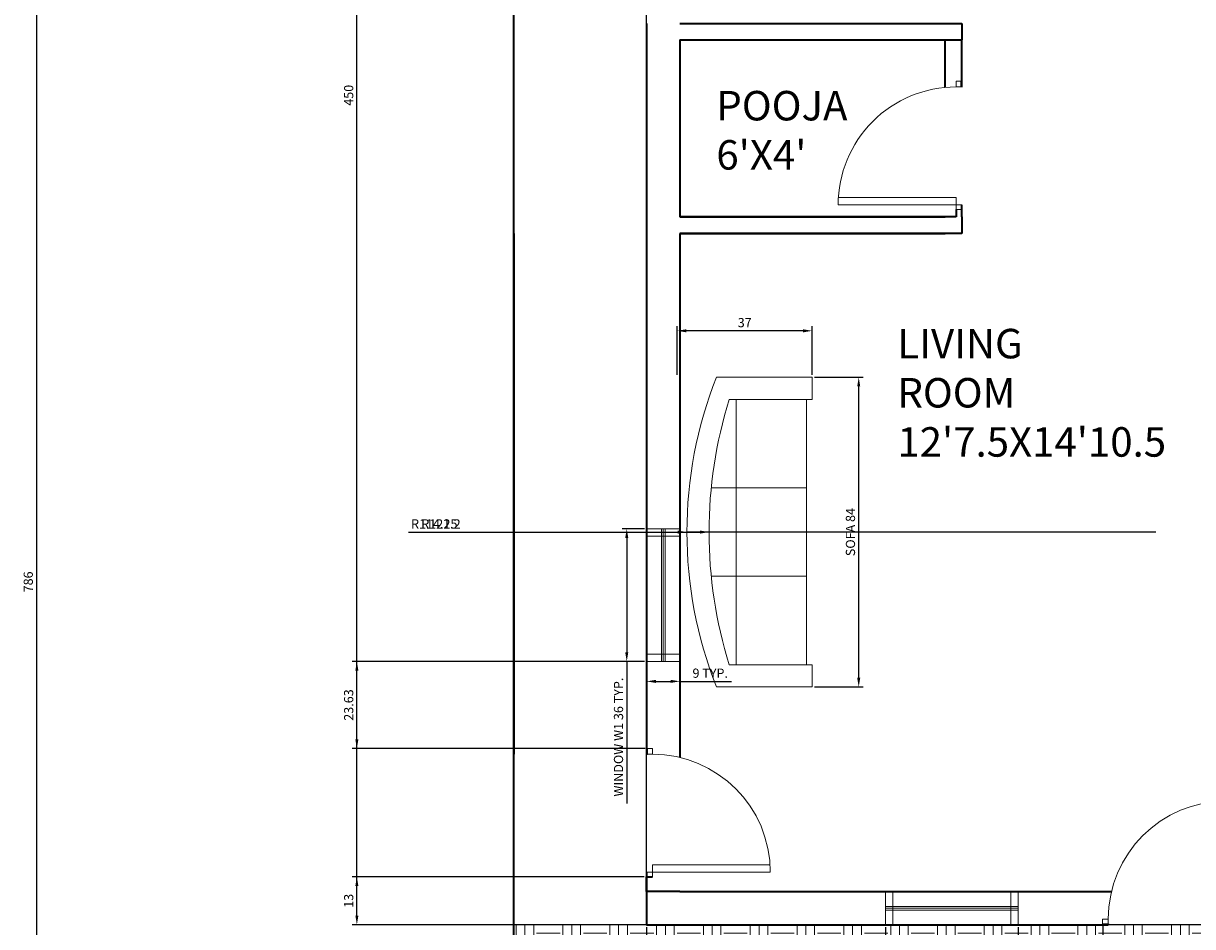
# Model space of a CAD drawing. Units: inches. Extents: x 204 to 942, y 1794 to 2670.
# Tile 3 of 6: x 204 to 521, y 2138 to 2383. Entities that reach past the tile are written whole.
import ezdxf

# ---------------------------------------------------------------- set-up
doc = ezdxf.new("R2010")
doc.units = ezdxf.units.IN
for name, color, linetype, lineweight in [('A-ANNO-DIMS', 2, 'Continuous', 18), ('A-AREA-IDEN', 7, 'Continuous', 18), ('A-DOOR', 3, 'Continuous', 18), ('A-FLOR-OTLN', 7, 'Continuous', 25), ('A-FURN', 8, 'Continuous', 18), ('A-GLAZ', 4, 'Continuous', 18), ('A-WALL', 7, 'Continuous', 35), ('C-PROP', 7, 'Continuous', 35)]:
    doc.layers.add(name, color=color, linetype=linetype, lineweight=lineweight)
doc.layers.add('A-FLOR-PATT', color=251, linetype='Continuous', lineweight=13, true_color=0x636466)
doc.styles.get("Standard").update_dxf_attribs({"font": 'arial.ttf'})
doc.dimstyles.new('ISO-25', dxfattribs={"dimtxt": 2.5, "dimasz": 2.5, "dimexe": 1.25, "dimexo": 0.625, "dimtad": 1, "dimtxsty": 'Standard', "dimcen": 2.5, "dimadec": 0, "dimazin": 0, "dimtfac": 1, "dimtmove": 0, "dimatfit": 3, "dimfxl": 1, "dimarcsym": 0})

# ---------------------------------------------------------------- blocks, each defined once
blk = doc.blocks.new('Sofa - Roundback 7 ft.')
for p, q in [((-12.00002, -32.4421), (-12.00003, -6.5971)), ((11.99997, -32.4421), (11.99998, -6.5971)), ((-36.000027, -34), (-36.000027, -11.4696)), ((35.99998, -34), (35.99998, -11.4696)), ((-35.999844, -13.3819), (35.9998, -13.3819)), ((-36.000027, -32.4421), (35.99998, -32.4421))]:
    blk.add_line(p, q)
for points in [[(-36.000027, -34), (-42.000027, -34), (-42.000027, -8)], [(41.99998, -8), (41.99998, -34), (35.99998, -34)]]:
    blk.add_lwpolyline(points)
for centre, radius, start, end in [((0, -114.25), 114.25, 68.43141, 111.5686), ((-0.00001, -127.1968), 121.1968, 72.72033, 107.2797)]:
    blk.add_arc(centre, radius, start, end)
blk = doc.blocks.new('*D11')
at = {"layer": 'A-ANNO-DIMS', "color": 0, "lineweight": -2, "transparency": 16777216}
for p, q in [((336.12, 2624.26), (205.97, 2624.26)), ((207.22, 2621.76), (207.22, 1840.76)), ((336.12, 1838.26), (205.97, 1838.26))]:
    blk.add_line(p, q, dxfattribs=at)
at = {"layer": 'A-ANNO-DIMS', "color": 0, "transparency": 16777216}
for points in [[(206.8, 2621.76), (207.63, 2621.76), (207.22, 2624.26)], [(206.8, 1840.76), (207.63, 1840.76), (207.22, 1838.26)]]:
    blk.add_solid(points, dxfattribs=at)
at = {"layer": 'Defpoints', "color": 0, "transparency": 16777216}
for p in [(336.74, 2624.26), (207.22, 1838.26), (336.74, 1838.26)]:
    blk.add_point(p, dxfattribs=at)
at = {"layer": 'A-ANNO-DIMS', "color": 0, "transparency": 16777216, "insert": (205.32, 2231.26), "char_height": 2.5, "attachment_point": 5, "rotation": 90}
blk.add_mtext('786', dxfattribs=at)
blk = doc.blocks.new('WIN-36IN')
for p, q in [((0, 9), (36, 9)), ((0, 0), (0, 9)), ((2, 0), (2, 9)), ((34, 0), (34, 9)), ((36, 9), (36, 0)), ((0, 5), (36, 5)), ((0, 4.5), (36, 4.5)), ((0, 4), (36, 4)), ((36, 0), (0, 0)), ((0, 0), (2, 0)), ((36, 0), (34, 0))]:
    blk.add_line(p, q)
blk = doc.blocks.new('DOOR-SWING-32IN')
for p, q in [((3.26, 1.55), (3.26, 33.49)), ((1.26, 1.55), (3.26, 1.55))]:
    blk.add_line(p, q)
blk.add_lwpolyline([(1.26, 33.55), (1.26, 1.55), (3.26, 1.55)])
for points in [[(1.26, 1.55), (0, 1.55), (0, 0), (1.26, 0)], [(33.26, 1.55), (34.79, 1.55), (34.79, 0.26), (33.26, 0.26)]]:
    blk.add_lwpolyline(points, close=True)
blk.add_arc((1.26, 1.55), 32, 0, 90)
blk = doc.blocks.new('*D18')
at = {"layer": 'A-ANNO-DIMS', "color": 0, "lineweight": -2, "transparency": 16777216}
for p, q in [((372.13, 2245.68), (366.1, 2245.68)), ((367.35, 2243.18), (367.35, 2212.18)), ((372.13, 2209.68), (366.1, 2209.68)), ((367.35, 2209.68), (367.35, 2171.15))]:
    blk.add_line(p, q, dxfattribs=at)
at = {"layer": 'A-ANNO-DIMS', "color": 0, "transparency": 16777216}
for points in [[(366.94, 2243.18), (367.77, 2243.18), (367.35, 2245.68)], [(366.94, 2212.18), (367.77, 2212.18), (367.35, 2209.68)]]:
    blk.add_solid(points, dxfattribs=at)
at = {"layer": 'Defpoints', "color": 0, "transparency": 16777216}
for p in [(372.75, 2245.68), (367.35, 2209.68), (372.75, 2209.68)]:
    blk.add_point(p, dxfattribs=at)
at = {"layer": 'A-ANNO-DIMS', "color": 0, "transparency": 16777216, "insert": (365.44, 2189.16), "char_height": 2.5, "attachment_point": 5, "rotation": 90}
blk.add_mtext('WINDOW W1 36 TYP.', dxfattribs=at)
blk = doc.blocks.new('*D19')
at = {"layer": 'A-ANNO-DIMS', "color": 0, "lineweight": -2, "transparency": 16777216}
for p, q in [((372.75, 2209.05), (372.75, 2203.03)), ((381.75, 2209.05), (381.75, 2203.03)), ((375.25, 2204.28), (379.25, 2204.28)), ((381.75, 2204.28), (395.73, 2204.28))]:
    blk.add_line(p, q, dxfattribs=at)
at = {"layer": 'A-ANNO-DIMS', "color": 0, "transparency": 16777216}
for points in [[(375.25, 2204.69), (375.25, 2203.86), (372.75, 2204.28)], [(379.25, 2204.69), (379.25, 2203.86), (381.75, 2204.28)]]:
    blk.add_solid(points, dxfattribs=at)
at = {"layer": 'Defpoints', "color": 0, "transparency": 16777216}
for p in [(372.75, 2209.68), (381.75, 2209.68), (381.75, 2204.28)]:
    blk.add_point(p, dxfattribs=at)
at = {"layer": 'A-ANNO-DIMS', "color": 0, "transparency": 16777216, "insert": (389.99, 2206.18), "char_height": 2.5, "attachment_point": 5}
blk.add_mtext('9 TYP.', dxfattribs=at)
blk = doc.blocks.new('*D34')
at = {"layer": 'A-ANNO-DIMS', "color": 0, "lineweight": -2, "transparency": 16777216}
for p, q in [((418.31, 2286.77), (431.53, 2286.77)), ((430.28, 2205.27), (430.28, 2284.27)), ((418.31, 2202.77), (431.53, 2202.77))]:
    blk.add_line(p, q, dxfattribs=at)
at = {"layer": 'A-ANNO-DIMS', "color": 0, "transparency": 16777216}
for points in [[(429.86, 2284.27), (430.7, 2284.27), (430.28, 2286.77)], [(429.86, 2205.27), (430.7, 2205.27), (430.28, 2202.77)]]:
    blk.add_solid(points, dxfattribs=at)
at = {"layer": 'Defpoints', "color": 0, "transparency": 16777216}
for p in [(417.68, 2286.77), (430.28, 2286.77), (417.68, 2202.77)]:
    blk.add_point(p, dxfattribs=at)
at = {"layer": 'A-ANNO-DIMS', "color": 0, "transparency": 16777216, "insert": (428.36, 2244.77), "char_height": 2.5, "attachment_point": 5, "rotation": 90}
blk.add_mtext('SOFA 84', dxfattribs=at)
blk = doc.blocks.new('*D35')
at = {"layer": 'A-ANNO-DIMS', "color": 0, "lineweight": -2, "transparency": 16777216}
for p, q in [((381.01, 2287.4), (381.01, 2300.62)), ((417.68, 2287.4), (417.68, 2300.62)), ((415.18, 2299.37), (383.51, 2299.37))]:
    blk.add_line(p, q, dxfattribs=at)
at = {"layer": 'A-ANNO-DIMS', "color": 0, "transparency": 16777216}
for points in [[(383.51, 2299.79), (383.51, 2298.95), (381.01, 2299.37)], [(415.18, 2299.79), (415.18, 2298.95), (417.68, 2299.37)]]:
    blk.add_solid(points, dxfattribs=at)
at = {"layer": 'Defpoints', "color": 0, "transparency": 16777216}
for p in [(381.01, 2299.37), (381.01, 2286.77), (417.68, 2286.77)]:
    blk.add_point(p, dxfattribs=at)
at = {"layer": 'A-ANNO-DIMS', "color": 0, "transparency": 16777216, "insert": (399.35, 2301.27), "char_height": 2.5, "attachment_point": 5}
blk.add_mtext('37', dxfattribs=at)
blk = doc.blocks.new('*D39')
at = {"layer": 'A-ANNO-DIMS', "color": 0, "lineweight": -2, "transparency": 16777216}
for p, q in [((372.12, 2588.26), (292.89, 2588.26)), ((294.14, 2140.76), (294.14, 2585.76)), ((336.12, 2138.26), (292.89, 2138.26))]:
    blk.add_line(p, q, dxfattribs=at)
at = {"layer": 'A-ANNO-DIMS', "color": 0, "transparency": 16777216}
for points in [[(293.73, 2585.76), (294.56, 2585.76), (294.14, 2588.26)], [(293.73, 2140.76), (294.56, 2140.76), (294.14, 2138.26)]]:
    blk.add_solid(points, dxfattribs=at)
at = {"layer": 'Defpoints', "color": 0, "transparency": 16777216}
for p in [(294.14, 2588.26), (372.74, 2588.26), (336.74, 2138.26)]:
    blk.add_point(p, dxfattribs=at)
at = {"layer": 'A-ANNO-DIMS', "color": 0, "transparency": 16777216, "insert": (292.24, 2363.26), "char_height": 2.5, "attachment_point": 5, "rotation": 90}
blk.add_mtext('450', dxfattribs=at)
blk = doc.blocks.new('*D54')
at = {"layer": 'A-ANNO-DIMS', "color": 0, "lineweight": -2, "transparency": 16777216}
for p, q in [((372.74, 2137.63), (372.74, 1794.41)), ((437.53, 2137.62), (437.53, 1794.41)), ((375.24, 1795.66), (435.03, 1795.66))]:
    blk.add_line(p, q, dxfattribs=at)
at = {"layer": 'A-ANNO-DIMS', "color": 0, "transparency": 16777216}
for points in [[(375.24, 1796.08), (375.24, 1795.24), (372.74, 1795.66)], [(435.03, 1796.08), (435.03, 1795.24), (437.53, 1795.66)]]:
    blk.add_solid(points, dxfattribs=at)
at = {"layer": 'Defpoints', "color": 0, "transparency": 16777216}
for p in [(372.74, 2138.26), (437.53, 2138.25), (437.53, 1795.66)]:
    blk.add_point(p, dxfattribs=at)
at = {"layer": 'A-ANNO-DIMS', "color": 0, "transparency": 16777216, "insert": (405.14, 1797.56), "char_height": 2.5, "attachment_point": 5}
blk.add_mtext('64.78', dxfattribs=at)
blk = doc.blocks.new('*D55')
at = {"layer": 'A-ANNO-DIMS', "color": 0, "lineweight": -2, "transparency": 16777216}
for p, q in [((496.46, 2137.89), (496.46, 1794.41)), ((473.53, 2137.62), (473.53, 1794.41)), ((476.03, 1795.66), (493.96, 1795.66))]:
    blk.add_line(p, q, dxfattribs=at)
at = {"layer": 'A-ANNO-DIMS', "color": 0, "transparency": 16777216}
for points in [[(476.03, 1796.08), (476.03, 1795.24), (473.53, 1795.66)], [(493.96, 1796.08), (493.96, 1795.24), (496.46, 1795.66)]]:
    blk.add_solid(points, dxfattribs=at)
at = {"layer": 'Defpoints', "color": 0, "transparency": 16777216}
for p in [(473.53, 2138.25), (496.46, 2138.52), (496.46, 1795.66)]:
    blk.add_point(p, dxfattribs=at)
at = {"layer": 'A-ANNO-DIMS', "color": 0, "transparency": 16777216, "insert": (484.99, 1797.56), "char_height": 2.5, "attachment_point": 5}
blk.add_mtext('22.93', dxfattribs=at)
blk = doc.blocks.new('*D57')
at = {"layer": 'A-ANNO-DIMS', "color": 0, "lineweight": -2, "transparency": 16777216}
for p, q in [((372.13, 2209.68), (292.89, 2209.68)), ((294.14, 2188.55), (294.14, 2207.18)), ((372.38, 2186.05), (292.89, 2186.05))]:
    blk.add_line(p, q, dxfattribs=at)
at = {"layer": 'A-ANNO-DIMS', "color": 0, "transparency": 16777216}
for points in [[(293.73, 2207.18), (294.56, 2207.18), (294.14, 2209.68)], [(293.73, 2188.55), (294.56, 2188.55), (294.14, 2186.05)]]:
    blk.add_solid(points, dxfattribs=at)
at = {"layer": 'Defpoints', "color": 0, "transparency": 16777216}
for p in [(294.14, 2209.68), (372.75, 2209.68), (373, 2186.05)]:
    blk.add_point(p, dxfattribs=at)
at = {"layer": 'A-ANNO-DIMS', "color": 0, "transparency": 16777216, "insert": (292.24, 2197.86), "char_height": 2.5, "attachment_point": 5, "rotation": 90}
blk.add_mtext('23.63', dxfattribs=at)
blk = doc.blocks.new('*D58')
at = {"layer": 'A-ANNO-DIMS', "color": 0, "lineweight": -2, "transparency": 16777216}
for p, q in [((372.12, 2151.26), (292.89, 2151.26)), ((294.14, 2140.76), (294.14, 2148.76)), ((372.12, 2138.26), (292.89, 2138.26))]:
    blk.add_line(p, q, dxfattribs=at)
at = {"layer": 'A-ANNO-DIMS', "color": 0, "transparency": 16777216}
for points in [[(293.73, 2148.76), (294.56, 2148.76), (294.14, 2151.26)], [(293.73, 2140.76), (294.56, 2140.76), (294.14, 2138.26)]]:
    blk.add_solid(points, dxfattribs=at)
at = {"layer": 'Defpoints', "color": 0, "transparency": 16777216}
for p in [(294.14, 2151.26), (372.74, 2151.26), (372.74, 2138.26)]:
    blk.add_point(p, dxfattribs=at)
at = {"layer": 'A-ANNO-DIMS', "color": 0, "transparency": 16777216, "insert": (292.24, 2144.76), "char_height": 2.5, "attachment_point": 5, "rotation": 90}
blk.add_mtext('13', dxfattribs=at)
blk = doc.blocks.new('*D64')
at = {"layer": 'A-ANNO-DIMS', "color": 0, "lineweight": -2, "transparency": 16777216}
for p, q in [((310.94, 2244.77), (387.18, 2244.77)), ((510.88, 2244.77), (389.68, 2244.77))]:
    blk.add_line(p, q, dxfattribs=at)
at = {"layer": 'A-ANNO-DIMS', "color": 0, "transparency": 16777216}
blk.add_solid([(387.18, 2245.19), (387.18, 2244.35), (389.68, 2244.77)], dxfattribs=at)
at = {"layer": 'Defpoints', "color": 0, "transparency": 16777216}
for p in [(389.68, 2244.77), (510.88, 2244.77)]:
    blk.add_point(p, dxfattribs=at)
at = {"layer": 'A-ANNO-DIMS', "color": 0, "transparency": 16777216, "insert": (316.96, 2246.65), "char_height": 2.5, "attachment_point": 5, "rotation": 0.0002}
blk.add_mtext('R121.2', dxfattribs=at)
blk = doc.blocks.new('*D65')
at = {"layer": 'A-ANNO-DIMS', "color": 0, "lineweight": -2, "transparency": 16777216}
for p, q in [((308.11, 2244.77), (381.18, 2244.77)), ((497.93, 2244.77), (383.68, 2244.77))]:
    blk.add_line(p, q, dxfattribs=at)
at = {"layer": 'A-ANNO-DIMS', "color": 0, "transparency": 16777216}
blk.add_solid([(381.18, 2245.19), (381.18, 2244.35), (383.68, 2244.77)], dxfattribs=at)
at = {"layer": 'Defpoints', "color": 0, "transparency": 16777216}
for p in [(383.68, 2244.77), (497.93, 2244.77)]:
    blk.add_point(p, dxfattribs=at)
at = {"layer": 'A-ANNO-DIMS', "color": 0, "transparency": 16777216, "insert": (315.13, 2246.67), "char_height": 2.5, "attachment_point": 5, "rotation": 0.0002}
blk.add_mtext('R114.25', dxfattribs=at)

msp = doc.modelspace()

# ---------------------------------------------------------------- hatches: boundary and pattern name
at = {"layer": 'A-FLOR-PATT'}
h = msp.add_hatch(dxfattribs=at)
h.set_pattern_fill('EARTH', color=256)
h.paths.add_polyline_path([(533.8633, 2137.2597), (533.8633, 2138.2597), (473.5284, 2138.2597), (473.5284, 2138.2472), (471.5284, 2138.2472), (437.5284, 2138.2472), (372.7443, 2138.2597), (336.7443, 2138.2597), (336.7443, 2014.1774), (533.8633, 2014.1774)])

# ---------------------------------------------------------------- linework, layer by layer
at = {"layer": 'A-FLOR-OTLN'}
for p, q in [((372.7443, 2138.2597), (336.7443, 2138.2597)), ((336.7443, 2138.2597), (336.7443, 2014.1774))]:
    msp.add_line(p, q, dxfattribs=at)
msp.add_lwpolyline([(372.7443, 2588.2597), (690.7443, 2588.2597), (690.7443, 2138.2597), (372.7443, 2138.2597)], close=True, dxfattribs=at)
at = {"layer": 'A-GLAZ'}
for p, q in [((437.5284, 2147.2472), (473.5284, 2147.2472)), ((437.5284, 2138.2472), (437.5284, 2147.2472)), ((439.5284, 2138.2472), (439.5284, 2147.2472)), ((471.5284, 2138.2472), (471.5284, 2147.2472)), ((473.5284, 2147.2472), (473.5284, 2138.2472)), ((437.5284, 2143.2472), (473.5284, 2143.2472)), ((437.5284, 2142.7472), (473.5284, 2142.7472)), ((437.5284, 2142.2472), (473.5284, 2142.2472)), ((473.5284, 2138.2472), (437.5284, 2138.2472)), ((437.5284, 2138.2472), (439.5284, 2138.2472)), ((473.5284, 2138.2472), (471.5284, 2138.2472))]:
    msp.add_line(p, q, dxfattribs=at)
at = {"layer": 'A-WALL'}
for p, q in [((372.7443, 2382.7597), (372.7443, 2325.7597)), ((381.7443, 2382.7597), (458.2443, 2382.7597)), ((458.2443, 2382.7597), (458.2443, 2378.2597)), ((381.7443, 2378.2597), (458.2443, 2378.2597)), ((381.7443, 2378.2597), (381.7443, 2330.2597)), ((453.7443, 2365.3856), (453.7443, 2378.2597)), ((458.2443, 2365.4841), (458.2443, 2378.2597)), ((456.6928, 2332.2597), (456.6928, 2330.2597)), ((458.2443, 2330.2597), (458.2443, 2333.5218)), ((458.2443, 2330.2597), (458.2443, 2332.2597)), ((381.7443, 2330.2597), (453.7443, 2330.2597)), ((456.6928, 2330.2597), (381.7443, 2330.2597)), ((458.2443, 2330.2597), (458.2443, 2325.7597)), ((372.7443, 2325.7597), (372.7443, 2184.5218)), ((381.7443, 2325.7597), (453.7443, 2325.7597)), ((381.7443, 2325.7597), (381.7443, 2183.6428)), ((458.2443, 2325.7597), (381.7443, 2325.7597)), ((373.0001, 2184.5218), (372.7443, 2184.5218)), ((372.7443, 2152.5218), (372.7443, 2138.2597)), ((372.7443, 2149.2597), (372.7443, 2151.2597)), ((372.7443, 2151.2597), (374.2958, 2151.2597)), ((372.7443, 2147.2597), (372.7443, 2149.2597)), ((381.7443, 2147.2597), (372.7443, 2147.2597)), ((381.7443, 2147.2597), (498.8612, 2147.2597)), ((372.7443, 2138.2597), (497.9822, 2138.2597)), ((497.9822, 2138.5155), (497.9822, 2138.2597))]:
    msp.add_line(p, q, dxfattribs=at)
at = {"layer": 'C-PROP'}
msp.add_line((336.7443, 2325.7597), (336.7443, 2184.5218), dxfattribs=at)
msp.add_lwpolyline([(336.7443, 2102.2597), (336.7443, 2624.2597), (726.7443, 2624.2597), (726.7443, 2102.2597)], dxfattribs=at)

# ---------------------------------------------------------------- block references
at = {"layer": 'A-DOOR', "rotation": 89.99999999999913}
msp.add_blockref('DOOR-SWING-32IN', (458.244, 2332.2594), dxfattribs=at)
at = {"layer": 'A-DOOR', "extrusion": (0, 0, -1), "zscale": -1, "rotation": 90.00000000000072}
msp.add_blockref('DOOR-SWING-32IN', (-372.7446, 2151.2594), dxfattribs=at)
at = {"layer": 'A-DOOR', "extrusion": (0, 0, -1), "zscale": -1}
msp.add_blockref('DOOR-SWING-32IN', (-531.2446, 2138.26), dxfattribs=at)
at = {"layer": 'A-FURN', "rotation": 90}
msp.add_blockref('Sofa - Roundback 7 ft.', (383.6815, 2244.7713), dxfattribs=at)
at = {"layer": 'A-GLAZ', "rotation": 269.9999999999978}
msp.add_blockref('WIN-36IN', (372.7542, 2245.6753), dxfattribs=at)

# ---------------------------------------------------------------- texts
at = {"layer": 'A-AREA-IDEN', "char_height": 2.5, "attachment_point": 1}
for s, insert in [("{\\H3.2x;POOJA\\P6'X4' }", (391.6608, 2364.4354)), ("{\\H3.2x;LIVING ROOM\\P12'7.5X14'10.5 }", (440.7643, 2299.8977))]:
    msp.add_mtext_dynamic_manual_height_columns(s, width=46.676204, gutter_width=12.5, heights=[0], dxfattribs=dict(at, insert=insert))

# ---------------------------------------------------------------- dimensions: what is measured, and where the dimension line sits
at = {"layer": 'A-ANNO-DIMS'}
for base, p1, p2, angle, override, picture, middle in [((207.2181, 1838.2597), (336.7443, 2624.2597), (336.7443, 1838.2597), 90, {"dimclrd": 0, "dimclre": 0, "dimclrt": 0}, '*D11', (205.3166, 2231.2597)), ((294.1443, 2588.2597), (336.7443, 2138.2597), (372.7443, 2588.2597), 90, {"dimdec": 0, "dimlfac": 1, "dimrnd": 0, "dimzin": 0, "dimdsep": 46, "dimlunit": 2}, '*D39', (292.2429, 2363.2597)), ((381.0148, 2299.3713), (417.6815, 2286.7713), (381.0148, 2286.7713), 180, {"dimdec": 0, "dimlfac": 1, "dimrnd": 0, "dimzin": 0, "dimdsep": 46, "dimlunit": 2}, '*D35', (399.3482, 2301.2736)), ((294.1443, 2209.6758), (373.0001, 2186.0453), (372.7543, 2209.6758), 90, {"dimdec": 2, "dimlfac": 1, "dimrnd": 0, "dimzin": 0, "dimdsep": 46, "dimlunit": 2}, '*D57', (292.242, 2197.8606)), ((294.1443, 2151.2597), (372.7443, 2138.2597), (372.7443, 2151.2597), 90, {"dimdec": 0, "dimlfac": 1, "dimrnd": 0, "dimzin": 0, "dimdsep": 46, "dimlunit": 2}, '*D58', (292.242, 2144.7597))]:
    dim = msp.add_linear_dim(base=base, p1=p1, p2=p2, angle=angle, dimstyle='ISO-25', override=override, dxfattribs=at)
    dim.commit()
    dim.dimension.update_dxf_attribs({"geometry": picture, "text_midpoint": middle})
for base, p1, p2, angle, text, picture, middle in [((430.2815, 2286.7713), (417.6815, 2202.7713), (417.6815, 2286.7713), 90, 'SOFA <>', '*D34', (428.363, 2244.7713)), ((367.3543, 2209.6758), (372.7543, 2245.6758), (372.7543, 2209.6758), 270, 'WINDOW W1 <> TYP.', '*D18', (365.435, 2189.1634))]:
    dim = msp.add_linear_dim(base=base, p1=p1, p2=p2, angle=angle, text=text, dimstyle='ISO-25', override={"dimdec": 0, "dimlfac": 1, "dimrnd": 0, "dimzin": 0, "dimdsep": 46, "dimlunit": 2}, dxfattribs=at)
    dim.commit()
    dim.dimension.update_dxf_attribs({"geometry": picture, "text_midpoint": middle})
for center, mpoint, override, picture, middle in [((497.9315, 2244.7713), (383.6815, 2244.771), {"dimdec": 2, "dimlfac": 1, "dimrnd": 0, "dimzin": 0, "dimdsep": 46, "dimlunit": 2}, '*D65', (315.1315, 2244.7708)), ((510.8783, 2244.7713), (389.6815, 2244.771), {"dimdec": 1, "dimlfac": 1, "dimrnd": 0, "dimzin": 0, "dimdsep": 46, "dimlunit": 2}, '*D64', (316.9634, 2244.7708))]:
    dim = msp.add_radius_dim(center=center, mpoint=mpoint, dimstyle='ISO-25', override=override, dxfattribs=at)
    dim.commit()
    dim.dimension.update_dxf_attribs({"geometry": picture, "text_midpoint": middle, "dimtype": 164})
dim = msp.add_linear_dim(base=(381.7543, 2204.2758), p1=(372.7543, 2209.6758), p2=(381.7543, 2209.6758), text='<> TYP.', dimstyle='ISO-25', override={"dimdec": 0, "dimlfac": 1, "dimrnd": 0, "dimzin": 0, "dimdsep": 46, "dimlunit": 2}, dxfattribs=at)
dim.commit()
dim.dimension.update_dxf_attribs({"geometry": '*D19', "text_midpoint": (389.9927, 2206.1773)})
for base, p1, p2, picture, middle in [((437.5284, 1795.6597), (372.7443, 2138.2597), (437.5284, 2138.2472), '*D54', (405.1364, 1797.5611)), ((496.4586, 1795.6597), (473.5284, 2138.2472), (496.4586, 2138.5155), '*D55', (484.9935, 1797.5619))]:
    dim = msp.add_linear_dim(base=base, p1=p1, p2=p2, dimstyle='ISO-25', override={"dimdec": 2, "dimlfac": 1, "dimrnd": 0, "dimzin": 0, "dimdsep": 46, "dimlunit": 2}, dxfattribs=at)
    dim.commit()
    dim.dimension.update_dxf_attribs({"geometry": picture, "text_midpoint": middle})

doc.saveas('drawing.dxf')
